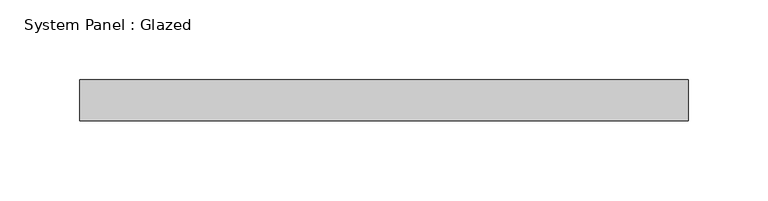
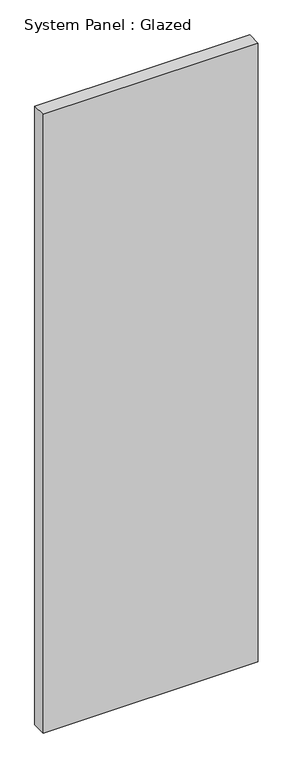
"""IFC4 building model written with IfcOpenShell, lengths in millimetres: plate geometry, System Panel : Glazed."""

from ifc_helpers import new_model, si_unit, origin, origin_with_axes, place, context, project, spatial, polyline, outline, extrude, source, transform, mapped, element, save


def system_panel_glazed_c821ef0e(model_context):
    return source(origin(), model_context, "Body", "SweptSolid", [
        extrude(outline(polyline([(190.0597519, 19.05), (-190.0597519, 19.05), (-190.0597519, 44.45), (190.0597519, 44.45), (190.0597519, 19.05)])), origin_with_axes(), (0.0, 0.0, 1.0), 1155.7),
    ])


if __name__ == "__main__":
    model = new_model("IFC4")
    model_context = context("Model", 3, world=origin())
    ifc_project = project(units=[si_unit("LENGTHUNIT", "METRE", prefix="MILLI")], contexts=[model_context])
    site = spatial("IfcSite", under=ifc_project)
    building = spatial("IfcBuilding", under=site)
    placement = place(None, origin())
    system_panel_glazed_shape = system_panel_glazed_c821ef0e(model_context)
    element("IfcPlate", 1, ObjectType="System Panel : Glazed", at=placement, inside=building, context=model_context, shape_type="MappedRepresentation", body=[
        mapped(system_panel_glazed_shape, transform((0.0, 0.0, 0.0), x_axis=(1.0, 0.0, 0.0), y_axis=(0.0, 1.0, 0.0), z_axis=(0.0, 0.0, 1.0))),
    ])
    save(model, "model.ifc")

# Revit data of these elements
# Type "System Panel : Glazed"
#   Construction Type Id = "GSP4R"
#   Analytic Construction = "1/8 in Pilkington single glazing"
#   Visual Light Transmittance = 0.9
#   Solar Heat Gain Coefficient = 0.86
#   Heat Transfer Coefficient (U) = 1.18115 BTU/(h·ft²·°F)
# Element 1 (IfcPlate, "System Panel : Glazed")
#   Materials on its faces: "Glass"
# Materials
#   "Glass": class "Glass", colour RGB 0 128 192, transparency 0.75, Description = "Soda Lime Glass", Cost = 0
